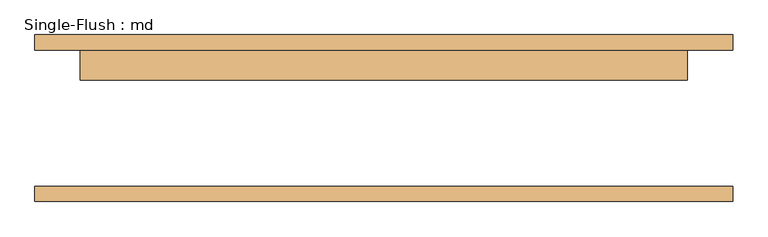
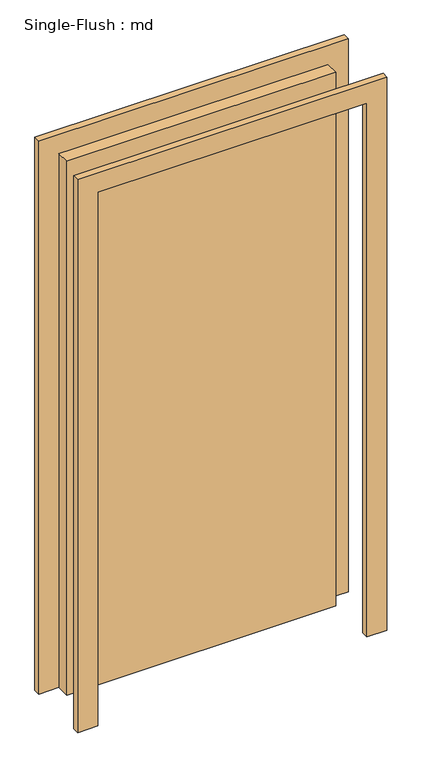
"""IFC4 building model written with IfcOpenShell, lengths in millimetres: door geometry, Single-Flush : md."""

from ifc_helpers import new_model, si_unit, frame, origin, origin_with_axes, place, context, project, spatial, polyline, outline, extrude, source, transform, mapped, element, save


def single_flush_md_00354a0c(model_context):
    return source(origin(), model_context, "Body", "SweptSolid", [
        extrude(outline(polyline([(2209.8, -584.2), (0.0, -584.2), (0.0, -508.0), (2133.6, -508.0), (2133.6, 508.0), (0.0, 508.0), (0.0, 584.2), (2209.8, 584.2), (2209.8, -584.2)])), frame((0.0, 114.3, 0.0), z_axis=(0.0, 1.0, 0.0), x_axis=(0.0, 0.0, 1.0)), (0.0, 0.0, 1.0), 25.4),
        extrude(outline(polyline([(2209.8, 584.2), (2209.8, -584.2), (0.0, -584.2), (0.0, -508.0), (2133.6, -508.0), (2133.6, 508.0), (0.0, 508.0), (0.0, 584.2), (2209.8, 584.2)])), frame((0.0, -139.7, 0.0), z_axis=(0.0, 1.0, 0.0), x_axis=(0.0, 0.0, 1.0)), (0.0, 0.0, 1.0), 25.4),
        extrude(outline(polyline([(508.0, 63.5), (-508.0, 63.5), (-508.0, 114.3), (508.0, 114.3), (508.0, 63.5)])), origin_with_axes(), (0.0, 0.0, 1.0), 2133.6),
    ])


if __name__ == "__main__":
    model = new_model("IFC4")
    model_context = context("Model", 3, world=origin())
    ifc_project = project(units=[si_unit("LENGTHUNIT", "METRE", prefix="MILLI")], contexts=[model_context])
    site = spatial("IfcSite", under=ifc_project)
    building = spatial("IfcBuilding", under=site)
    placement = place(None, origin())
    single_flush_md_shape = single_flush_md_00354a0c(model_context)
    element("IfcDoor", 1, ObjectType="Single-Flush : md", at=placement, inside=building, context=model_context, shape_type="MappedRepresentation", body=[
        mapped(single_flush_md_shape, transform((0.0, 0.0, 0.0), x_axis=(1.0, 0.0, 0.0), y_axis=(0.0, 1.0, 0.0), z_axis=(0.0, 0.0, 1.0))),
    ])
    save(model, "model.ifc")

# Revit data of these elements
# Type "Single-Flush : md"
#   Type Mark = "8"
#   Construction Type Id = "MDOOR"
#   Assembly Code = "C1020"
#   Analytic Construction = "Metal"
#   Thickness = 0' - 2"
#   Heat Transfer Coefficient (U) = 0.651978 BTU/(h·ft²·°F)
#   Height = 7' - 0"
#   Trim Projection Ext = 0' - 1"
#   Trim Projection Int = 0' - 1"
#   Trim Width = 0' - 3"
#   Width = 3' - 4"
#   Define Thermal Properties by = 1
#   Door Material = Door - Panel
#   Frame Material = Door - Frame
#   Visual Light Transmittance = 0
#   Solar Heat Gain Coefficient = 0
#   Function = (empty or 0)
#   Wall Closure = (empty or 0)
# Element 1 (IfcDoor, "Single-Flush : md")
#   Materials on its faces: "Door - Frame", "Door - Panel"
# Materials
#   "Door - Panel": class "Wood", colour RGB 210 159 95, transparency 0, Cost = 0
#   "Door - Frame": colour RGB 118 70 51, transparency 0, Cost = 0
